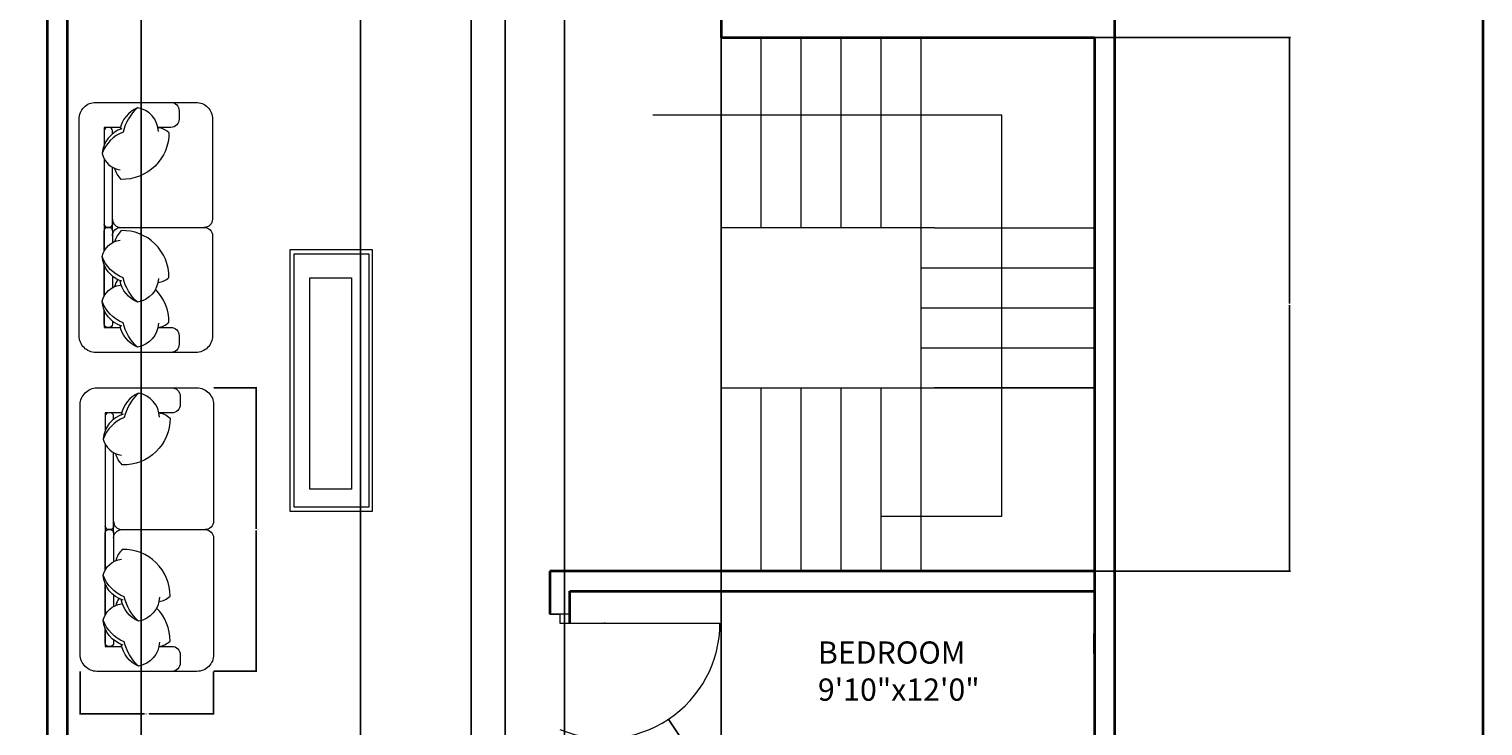
# Model space of a CAD drawing. Units: inches. Extents: x 1734 to 2405, y 1500 to 2491.
# Tile 10 of 14: x 2078 to 2405, y 1922 to 2078. Entities that reach past the tile are written whole.
import ezdxf

# ---------------------------------------------------------------- set-up
doc = ezdxf.new("R2010")
doc.units = ezdxf.units.IN
for name, color, linetype, lineweight in [('A-ANNO-DIMS', 2, 'Continuous', 18), ('A-ANNO-TTLB', 7, 'Continuous', 35), ('A-AREA-IDEN', 7, 'Continuous', 18), ('A-DOOR', 3, 'Continuous', 18), ('A-FLOR-STRS', 7, 'Continuous', 18), ('A-FURN', 8, 'Continuous', 13), ('A-WALL', 7, 'Continuous', 35)]:
    doc.layers.add(name, color=color, linetype=linetype, lineweight=lineweight)
doc.styles.get("Standard").update_dxf_attribs({"font": 'arial.ttf'})
doc.dimstyles.get("Standard").update_dxf_attribs({"dimtxt": 0.18, "dimasz": 0.18, "dimexe": 0.18, "dimexo": 0.0625, "dimgap": 0.09, "dimtad": 0, "dimtih": 1, "dimtoh": 1, "dimdec": 4, "dimzin": 0, "dimdsep": 46, "dimtxsty": 'Standard', "dimcen": 0.09, "dimadec": 0, "dimazin": 0, "dimtfac": 1, "dimtdec": 4, "dimtofl": 0, "dimtmove": 0, "dimatfit": 3, "dimfxl": 1, "dimtolj": 1, "dimtzin": 0, "dimarcsym": 0})

# ---------------------------------------------------------------- blocks, each defined once
blk = doc.blocks.new('SOFA-COMPACT')
at = {"ltscale": 0.03}
blk.add_lwpolyline([(29.99, 29.99, -0.414214), (28.12, 28.12, -0.414214), (29.99, 26.24), (29.99, 3.75, -0.414214), (26.24, 0), (3.75, 0, -0.414214), (0, 3.75), (0, 52.49, -0.414214), (3.75, 56.24), (26.24, 56.24, -0.414214), (29.99, 52.49), (29.99, 29.99, -0.414214), (28.12, 28.12, -0.414214), (29.99, 26.24)], format="xyb", dxfattribs=at)
for points in [[(20.62, 56.24, -0.414214), (22.49, 54.36), (22.49, 52.49, -0.414214), (20.62, 50.61), (17.72, 50.61)], [(13.1, 55.04, 0.14773), (9.88, 49.56, 0.213343), (5.16, 44.73, 0.178662)], [(17.83, 49.67, 0.356772), (13.1, 55.04, 0.249542), (9.21, 50.18, -9.61688)], [(9.63, 50.32, 0.306663), (5.16, 44.73, 0.30633), (9.24, 41.08, -0.872847)], [(7.5, 49.18), (7.5, 49.86, 0.414214), (6.75, 50.61), (6.37, 50.61, 0.414214), (5.62, 49.86)], [(5.62, 49.86), (5.62, 46.67, 0.414214)], [(17.71, 50.62, -0.165541), (20.19, 49.46, -0.425989), (9.45, 38.93, -0.121523), (7.97, 41.43, 7.115464)], [(5.62, 43.55), (5.62, 28.87, 0.414214), (6.37, 28.12), (6.75, 28.12, 0.414214), (7.5, 28.87), (7.5, 41.66, 0.414214)], [(7.5, 29.99, 0.414214), (9.37, 28.12)], [(7.5, 29.99, 0.414214), (9.37, 28.12), (28.12, 28.12, 0.414214)], [(5.62, 22.78), (5.62, 27.37, -0.414214), (6.37, 28.12), (6.75, 28.12, -0.414214), (7.5, 27.37), (7.5, 24.67, -0.414214)], [(7.5, 26.24, -0.414214), (9.37, 28.12)], [(7.5, 26.24, -0.414214), (9.37, 28.12), (28.12, 28.12, -0.414214)], [(17.71, 15.72, 0.165541), (20.19, 16.88, 0.425989), (9.45, 27.4, 0.121523), (7.97, 24.91, -7.115464)], [(9.63, 16.01, -0.306663), (5.16, 21.6, -0.30633), (9.24, 25.26, 0.872847)], [(13.1, 11.29, -0.14773), (9.88, 16.77, -0.213343), (5.16, 21.6, -0.178662)], [(5.62, 12.69), (5.62, 19.67, -0.414214)], [(7.5, 17.15), (7.5, 14.57, -0.414214)], [(8.71, 16.38, 0.071865), (7.97, 14.81, -7.115464)], [(17.83, 16.66, -0.356772), (13.1, 11.29, -0.249542), (9.21, 16.16, 9.61688)], [(9.63, 5.91, -0.306663), (5.16, 11.51, -0.30633), (9.24, 15.16, 0.872847)], [(17.71, 5.62, 0.165541), (20.19, 6.78, 0.200231), (17.17, 14.22, 0.121523)], [(13.1, 1.19, -0.14773), (9.88, 6.67, -0.213343), (5.16, 11.51, -0.178662)], [(5.62, 6.37), (5.62, 9.57, -0.414214)], [(5.62, 9.57), (5.62, 5.62), (9.31, 5.62, -0.414214)], [(7.5, 7.05), (7.5, 6.37, -0.414214), (6.75, 5.62), (6.37, 5.62, -0.414214), (5.62, 6.37)], [(17.83, 6.56, -0.356772), (13.1, 1.19, -0.249542), (9.21, 6.06, 9.61688)], [(17.72, 5.62), (20.62, 5.62, -0.414214), (22.49, 3.75), (22.49, 1.87, -0.414214), (20.62, 0)]]:
    blk.add_lwpolyline(points, format="xyb")
for points in [[(9.31, 50.61), (5.62, 50.61), (5.62, 46.67)], [(5.62, 43.55), (5.62, 22.78)], [(5.62, 19.67), (5.62, 12.69)]]:
    blk.add_lwpolyline(points)
blk.add_lwpolyline([(5.62, 28.87), (5.62, 27.37, -0.414214), (6.37, 28.12), (6.75, 28.12, -0.414214), (7.5, 27.37), (7.5, 28.87, -0.414214), (6.75, 28.12), (6.37, 28.12, -0.414214)], format="xyb", close=True)
blk = doc.blocks.new('SOFA-LONG')
at = {"ltscale": 0.03}
blk.add_lwpolyline([(29.99, 33.74, -0.414214), (28.12, 31.87, -0.414214), (29.99, 29.99), (29.99, 3.75, -0.414214), (26.24, 0), (3.75, 0, -0.414214), (0, 3.75), (0, 59.98, -0.414214), (3.75, 63.73), (26.24, 63.73, -0.414214), (29.99, 59.98), (29.99, 33.74, -0.414214), (28.12, 31.87, -0.414214), (29.99, 29.99)], format="xyb", dxfattribs=at)
for points in [[(13.1, 62.54, 0.14773), (9.88, 57.06, 0.213343), (5.16, 52.23, 0.178662)], [(17.83, 57.17, 0.356772), (13.1, 62.54, 0.249542), (9.21, 57.67, -9.61688)], [(20.62, 63.73, -0.414214), (22.49, 61.86), (22.49, 59.98, -0.414214), (20.62, 58.11), (17.71, 58.11)], [(9.63, 57.82, 0.306663), (5.16, 52.23, 0.30633), (9.24, 48.58, -0.872847)], [(7.5, 56.68), (7.5, 57.36, 0.414214), (6.75, 58.11), (6.37, 58.11, 0.414214), (5.62, 57.36)], [(5.62, 57.36), (5.62, 54.17, 0.414214)], [(17.71, 58.11, -0.165541), (20.19, 56.95, -0.425989), (9.45, 46.43, -0.121523), (7.97, 48.93, 7.115464)], [(5.62, 51.05), (5.62, 32.62, 0.414214), (6.37, 31.87), (6.75, 31.87, 0.414214), (7.5, 32.62), (7.5, 49.16, 0.414214)], [(7.5, 33.74, 0.414214), (9.37, 31.87)], [(7.5, 33.74, 0.414214), (9.37, 31.87), (28.12, 31.87, 0.414214)], [(5.62, 22.78), (5.62, 31.12, -0.414214), (6.37, 31.87), (6.75, 31.87, -0.414214), (7.5, 31.12), (7.5, 24.67, -0.414214)], [(7.5, 29.99, -0.414214), (9.37, 31.87)], [(7.5, 29.99, -0.414214), (9.37, 31.87), (28.12, 31.87, -0.414214)], [(17.71, 15.72, 0.165541), (20.19, 16.88, 0.425989), (9.45, 27.4, 0.121523), (7.97, 24.91, -7.115464)], [(9.63, 16.01, -0.306663), (5.16, 21.6, -0.30633), (9.24, 25.26, 0.872847)], [(13.1, 11.29, -0.14773), (9.88, 16.77, -0.213343), (5.16, 21.6, -0.178662)], [(5.62, 12.69), (5.62, 19.67, -0.414214)], [(7.5, 17.15), (7.5, 14.57, -0.414214)], [(8.71, 16.38, 0.071865), (7.97, 14.81, -7.115464)], [(17.83, 16.66, -0.356772), (13.1, 11.29, -0.249542), (9.21, 16.16, 9.61688)], [(9.63, 5.92, -0.306663), (5.16, 11.51, -0.30633), (9.24, 15.16, 0.872847)], [(17.71, 5.62, 0.165541), (20.19, 6.78, 0.200231), (17.17, 14.22, 0.121523)], [(13.1, 1.19, -0.14773), (9.88, 6.67, -0.213343), (5.16, 11.51, -0.178662)], [(5.62, 9.57), (5.62, 5.62), (9.31, 5.62, -0.414214)], [(5.62, 6.37), (5.62, 9.57, -0.414214)], [(7.5, 7.05), (7.5, 6.37, -0.414214), (6.75, 5.62), (6.37, 5.62, -0.414214), (5.62, 6.37)], [(17.83, 6.56, -0.356772), (13.1, 1.19, -0.249542), (9.21, 6.06, 9.61688)], [(17.71, 5.62), (20.62, 5.62, -0.414214), (22.49, 3.75), (22.49, 1.87, -0.414214), (20.62, 0)]]:
    blk.add_lwpolyline(points, format="xyb")
for points in [[(9.31, 58.11), (5.62, 58.11), (5.62, 54.17)], [(5.62, 51.05), (5.62, 22.78)], [(5.62, 19.67), (5.62, 12.69)]]:
    blk.add_lwpolyline(points)
blk.add_lwpolyline([(5.62, 32.62), (5.62, 31.12, -0.414214), (6.37, 31.87), (6.75, 31.87, -0.414214), (7.5, 31.12), (7.5, 32.62, -0.414214), (6.75, 31.87), (6.37, 31.87, -0.414214)], format="xyb", close=True)
blk = doc.blocks.new('TABLE-COFFEE')
for points in [[(0, 58.87), (18.49, 58.87), (18.49, 0), (0, 0)], [(0.91, 57.96), (17.71, 57.96), (17.71, 0.97), (0.91, 0.97)], [(4.43, 52.52), (13.86, 52.52), (13.86, 5), (4.43, 5)]]:
    blk.add_lwpolyline(points, close=True)
blk = doc.blocks.new('*D14')
at = {"layer": 'A-ANNO-DIMS', "color": 0, "lineweight": -2, "transparency": 16777216}
for p, q in [((2119.21, 1997.52), (2128.88, 1997.52)), ((2128.7, 1997.34), (2128.7, 1965.84)), ((2128.7, 1933.97), (2128.7, 1965.47)), ((2119.21, 1933.79), (2128.88, 1933.79))]:
    blk.add_line(p, q, dxfattribs=at)
at = {"layer": 'A-ANNO-DIMS', "color": 0, "transparency": 16777216}
for points in [[(2128.67, 1997.34), (2128.73, 1997.34), (2128.7, 1997.52)], [(2128.67, 1933.97), (2128.73, 1933.97), (2128.7, 1933.79)]]:
    blk.add_solid(points, dxfattribs=at)
at = {"layer": 'Defpoints', "color": 0, "transparency": 16777216}
for p in [(2119.14, 1997.52), (2128.7, 1997.52), (2119.14, 1933.79)]:
    blk.add_point(p, dxfattribs=at)
at = {"layer": 'A-ANNO-DIMS', "color": 0, "transparency": 16777216, "insert": (2128.7, 1965.65), "char_height": 0.18, "attachment_point": 5}
blk.add_mtext('\\A1;SOFA 64 TYP.', dxfattribs=at)
blk = doc.blocks.new('*D15')
at = {"layer": 'A-ANNO-DIMS', "color": 0, "lineweight": -2, "transparency": 16777216}
for p, q in [((2089.15, 1933.73), (2089.15, 1924.05)), ((2119.14, 1933.73), (2119.14, 1924.05)), ((2089.33, 1924.23), (2103.62, 1924.23)), ((2118.96, 1924.23), (2104.68, 1924.23))]:
    blk.add_line(p, q, dxfattribs=at)
at = {"layer": 'A-ANNO-DIMS', "color": 0, "transparency": 16777216}
for points in [[(2089.33, 1924.26), (2089.33, 1924.2), (2089.15, 1924.23)], [(2118.96, 1924.26), (2118.96, 1924.2), (2119.14, 1924.23)]]:
    blk.add_solid(points, dxfattribs=at)
at = {"layer": 'Defpoints', "color": 0, "transparency": 16777216}
for p in [(2089.15, 1933.79), (2119.14, 1933.79), (2119.14, 1924.23)]:
    blk.add_point(p, dxfattribs=at)
at = {"layer": 'A-ANNO-DIMS', "color": 0, "transparency": 16777216, "insert": (2104.15, 1924.23), "char_height": 0.18, "attachment_point": 5}
blk.add_mtext('\\A1;30 TYP.', dxfattribs=at)
blk = doc.blocks.new('*D36')
at = {"layer": 'A-ANNO-DIMS', "color": 0, "lineweight": -2, "transparency": 16777216}
for p, q in [((2081.68, 2425.82), (2042.21, 2425.82)), ((2042.39, 2425.64), (2042.39, 2065.96)), ((2042.39, 1705.92), (2042.39, 2065.6)), ((2081.68, 1705.74), (2042.21, 1705.74))]:
    blk.add_line(p, q, dxfattribs=at)
at = {"layer": 'A-ANNO-DIMS', "color": 0, "transparency": 16777216}
for points in [[(2042.36, 2425.64), (2042.42, 2425.64), (2042.39, 2425.82)], [(2042.36, 1705.92), (2042.42, 1705.92), (2042.39, 1705.74)]]:
    blk.add_solid(points, dxfattribs=at)
at = {"layer": 'Defpoints', "color": 0, "transparency": 16777216}
for p in [(2042.39, 2425.82), (2081.74, 2425.82), (2081.74, 1705.74)]:
    blk.add_point(p, dxfattribs=at)
at = {"layer": 'A-ANNO-DIMS', "color": 0, "transparency": 16777216, "insert": (2042.39, 2065.78), "char_height": 0.18, "attachment_point": 5}
blk.add_mtext('\\A1;720.1', dxfattribs=at)
blk = doc.blocks.new('*D39')
at = {"layer": 'A-ANNO-DIMS', "color": 0, "lineweight": -2, "transparency": 16777216}
for p, q in [((2317.31, 2076.32), (2361.27, 2076.32)), ((2361.09, 2076.14), (2361.09, 2016.51)), ((2361.09, 1956.5), (2361.09, 2016.14)), ((2317.31, 1956.32), (2361.27, 1956.32))]:
    blk.add_line(p, q, dxfattribs=at)
at = {"layer": 'A-ANNO-DIMS', "color": 0, "transparency": 16777216}
for points in [[(2361.06, 2076.14), (2361.12, 2076.14), (2361.09, 2076.32)], [(2361.06, 1956.5), (2361.12, 1956.5), (2361.09, 1956.32)]]:
    blk.add_solid(points, dxfattribs=at)
at = {"layer": 'Defpoints', "color": 0, "transparency": 16777216}
for p in [(2317.24, 2076.32), (2361.09, 2076.32), (2317.24, 1956.32)]:
    blk.add_point(p, dxfattribs=at)
at = {"layer": 'A-ANNO-DIMS', "color": 0, "transparency": 16777216, "insert": (2361.09, 2016.32), "char_height": 0.18, "attachment_point": 5}
blk.add_mtext('\\A1;120', dxfattribs=at)
blk = doc.blocks.new('*D41')
at = {"layer": 'A-ANNO-DIMS', "color": 0, "lineweight": -2, "transparency": 16777216}
for p, q in [((2233.24, 1956.26), (2233.24, 1611.24)), ((2317.24, 1956.26), (2317.24, 1611.24)), ((2233.42, 1611.42), (2275.03, 1611.42)), ((2317.06, 1611.42), (2275.46, 1611.42))]:
    blk.add_line(p, q, dxfattribs=at)
at = {"layer": 'A-ANNO-DIMS', "color": 0, "transparency": 16777216}
for points in [[(2233.42, 1611.45), (2233.42, 1611.39), (2233.24, 1611.42)], [(2317.06, 1611.45), (2317.06, 1611.39), (2317.24, 1611.42)]]:
    blk.add_solid(points, dxfattribs=at)
at = {"layer": 'Defpoints', "color": 0, "transparency": 16777216}
for p in [(2233.24, 1956.32), (2317.24, 1956.32), (2317.24, 1611.42)]:
    blk.add_point(p, dxfattribs=at)
at = {"layer": 'A-ANNO-DIMS', "color": 0, "transparency": 16777216, "insert": (2275.24, 1611.42), "char_height": 0.18, "attachment_point": 5}
blk.add_mtext('\\A1;84', dxfattribs=at)
blk = doc.blocks.new('*D42')
at = {"layer": 'A-ANNO-DIMS', "color": 0, "lineweight": -2, "transparency": 16777216}
for p, q in [((2152.2, 2198.26), (2152.2, 1611.24)), ((2184.72, 2198.26), (2184.72, 1611.24)), ((2152.38, 1611.42), (2168, 1611.42)), ((2184.54, 1611.42), (2168.92, 1611.42))]:
    blk.add_line(p, q, dxfattribs=at)
at = {"layer": 'A-ANNO-DIMS', "color": 0, "transparency": 16777216}
for points in [[(2152.38, 1611.45), (2152.38, 1611.39), (2152.2, 1611.42)], [(2184.54, 1611.45), (2184.54, 1611.39), (2184.72, 1611.42)]]:
    blk.add_solid(points, dxfattribs=at)
at = {"layer": 'Defpoints', "color": 0, "transparency": 16777216}
for p in [(2152.2, 2198.32), (2184.72, 2198.32), (2184.72, 1611.42)]:
    blk.add_point(p, dxfattribs=at)
at = {"layer": 'A-ANNO-DIMS', "color": 0, "transparency": 16777216, "insert": (2168.46, 1611.42), "char_height": 0.18, "attachment_point": 5}
blk.add_mtext('\\A1;32.526', dxfattribs=at)
blk = doc.blocks.new('*D43')
at = {"layer": 'A-ANNO-DIMS', "color": 0, "lineweight": -2, "transparency": 16777216}
for p, q in [((2233.24, 2200.45), (2233.24, 1611.24)), ((2198.08, 2198.26), (2198.08, 1611.24)), ((2198.26, 1611.42), (2215.27, 1611.42)), ((2233.06, 1611.42), (2216.05, 1611.42))]:
    blk.add_line(p, q, dxfattribs=at)
at = {"layer": 'A-ANNO-DIMS', "color": 0, "transparency": 16777216}
for points in [[(2198.26, 1611.45), (2198.26, 1611.39), (2198.08, 1611.42)], [(2233.06, 1611.45), (2233.06, 1611.39), (2233.24, 1611.42)]]:
    blk.add_solid(points, dxfattribs=at)
at = {"layer": 'Defpoints', "color": 0, "transparency": 16777216}
for p in [(2233.24, 2200.51), (2198.08, 2198.32), (2233.24, 1611.42)]:
    blk.add_point(p, dxfattribs=at)
at = {"layer": 'A-ANNO-DIMS', "color": 0, "transparency": 16777216, "insert": (2215.66, 1611.42), "char_height": 0.18, "attachment_point": 5}
blk.add_mtext('\\A1;35.17', dxfattribs=at)
blk = doc.blocks.new('*D44')
at = {"layer": 'A-ANNO-DIMS', "color": 0, "lineweight": -2, "transparency": 16777216}
for p, q in [((2102.87, 2356.76), (2102.87, 1611.24)), ((2177.04, 2356.76), (2177.04, 1611.24)), ((2103.05, 1611.42), (2139.56, 1611.42)), ((2176.86, 1611.42), (2140.35, 1611.42))]:
    blk.add_line(p, q, dxfattribs=at)
at = {"layer": 'A-ANNO-DIMS', "color": 0, "transparency": 16777216}
for points in [[(2103.05, 1611.45), (2103.05, 1611.39), (2102.87, 1611.42)], [(2176.86, 1611.45), (2176.86, 1611.39), (2177.04, 1611.42)]]:
    blk.add_solid(points, dxfattribs=at)
at = {"layer": 'Defpoints', "color": 0, "transparency": 16777216}
for p in [(2102.87, 2356.82), (2177.04, 2356.82), (2177.04, 1611.42)]:
    blk.add_point(p, dxfattribs=at)
at = {"layer": 'A-ANNO-DIMS', "color": 0, "transparency": 16777216, "insert": (2139.96, 1611.42), "char_height": 0.18, "attachment_point": 5}
blk.add_mtext('\\A1;74.17', dxfattribs=at)
blk = doc.blocks.new('*D50')
at = {"layer": 'A-ANNO-DIMS', "color": 0, "lineweight": -2, "transparency": 16777216}
for p, q in [((2206.97, 1944.63), (2207.15, 1944.63)), ((2207.06, 1944.54), (2207.06, 1944.72)), ((2230.01, 1910.06), (2221.5, 1922.88)), ((2230.19, 1910.06), (2230.01, 1910.06))]:
    blk.add_line(p, q, dxfattribs=at)
at = {"layer": 'A-ANNO-DIMS', "color": 0, "transparency": 16777216}
blk.add_solid([(2221.53, 1922.89), (2221.48, 1922.86), (2221.4, 1923.03)], dxfattribs=at)
at = {"layer": 'Defpoints', "color": 0, "transparency": 16777216}
for p in [(2207.06, 1944.63), (2221.4, 1923.03)]:
    blk.add_point(p, dxfattribs=at)
at = {"layer": 'A-ANNO-DIMS', "color": 0, "transparency": 16777216, "insert": (2230.67, 1910.06), "char_height": 0.18, "attachment_point": 5}
blk.add_mtext('\\A1;R25.93', dxfattribs=at)

msp = doc.modelspace()

# ---------------------------------------------------------------- linework, layer by layer
at = {"layer": 'A-ANNO-TTLB'}
msp.add_lwpolyline([(1734.1307, 2491.1293), (2404.5589, 2491.1293), (2404.5589, 1500.293), (1734.1307, 1500.293)], close=True, dxfattribs=at)
at = {"layer": 'A-DOOR'}
for p, q in [((2199.2445, 1946.6313), (2194.7445, 1946.6313)), ((2194.7445, 1946.6313), (2196.9945, 1946.6313)), ((2196.9945, 1946.6313), (2196.9945, 1944.6313)), ((2196.9945, 1944.6313), (2232.9945, 1944.6313))]:
    msp.add_line(p, q, dxfattribs=at)
msp.add_arc((2207.0621, 1944.6313), 25.9324, 247.155856, 0, dxfattribs=at)
at = {"layer": 'A-FLOR-STRS'}
for p, q in [((2233.2445, 2033.5364), (2233.2445, 2076.3246)), ((2242.2445, 2033.5364), (2242.2445, 2076.3246)), ((2251.2445, 2033.5364), (2251.2445, 2076.3246)), ((2260.2445, 2033.5364), (2260.2445, 2076.3246)), ((2269.2445, 2033.5364), (2269.2445, 2076.3246)), ((2278.2445, 2033.5364), (2278.2445, 2076.3246)), ((2217.8883, 2058.9549), (2296.2999, 2058.9549)), ((2296.2999, 2058.9549), (2296.2999, 1968.6387)), ((2281.2445, 2033.5364), (2233.2445, 2033.5364)), ((2278.2445, 1956.3246), (2278.2445, 2033.5364)), ((2281.2445, 2033.5364), (2317.2445, 2033.5364)), ((2278.2445, 2024.5364), (2317.2445, 2024.5364)), ((2278.2445, 2015.5364), (2317.2445, 2015.5364)), ((2278.2445, 2006.5364), (2317.2445, 2006.5364)), ((2233.2445, 1997.5364), (2233.2445, 1956.3246)), ((2233.2445, 1961.5364), (2233.2445, 1997.5364)), ((2233.2445, 1997.5364), (2317.2445, 1997.5364)), ((2242.2445, 1956.3246), (2242.2445, 1997.5364)), ((2251.2445, 1956.3246), (2251.2445, 1997.5364)), ((2260.2445, 1956.3246), (2260.2445, 1997.5364)), ((2269.2445, 1956.3246), (2269.2445, 1997.5364)), ((2317.2445, 1997.5364), (2281.2445, 1997.5364)), ((2296.2999, 1968.6387), (2269.2445, 1968.6387))]:
    msp.add_line(p, q, dxfattribs=at)
at = {"layer": 'A-WALL'}
for p, q in [((2081.7445, 2425.8246), (2081.7445, 1705.7415)), ((2321.7445, 2425.8246), (2321.7445, 1922.2954)), ((2086.2445, 2198.3246), (2086.2445, 1900.8246)), ((2233.2445, 2080.8246), (2233.2445, 2076.3246)), ((2233.2445, 2076.3246), (2237.7445, 2076.3246)), ((2237.7445, 2076.3246), (2317.2445, 2076.3246)), ((2317.2445, 2076.3246), (2317.2445, 1807.8246)), ((2317.2445, 2076.3246), (2317.2445, 2067.8246)), ((2317.2445, 2076.3246), (2317.2445, 2067.8246)), ((2199.2445, 1956.3246), (2194.7445, 1956.3246)), ((2194.7445, 1956.3246), (2194.7445, 1946.6313)), ((2317.2445, 1956.3246), (2199.2445, 1956.3246)), ((2199.2445, 1951.8246), (2317.2445, 1951.8246)), ((2199.2445, 1944.6313), (2199.2445, 1951.8246)), ((2317.2445, 1937.8246), (2317.2445, 1942.3246)), ((2321.7445, 1922.2954), (2321.7445, 1798.8246))]:
    msp.add_line(p, q, dxfattribs=at)

# ---------------------------------------------------------------- block references
at = {"layer": 'A-FURN'}
for name, p in [('SOFA-COMPACT', (2088.9007, 2005.4886)), ('TABLE-COFFEE', (2136.3236, 1969.7433)), ('SOFA-LONG', (2089.1527, 1933.7876))]:
    msp.add_blockref(name, p, dxfattribs=at)

# ---------------------------------------------------------------- texts
at = {"layer": 'A-AREA-IDEN', "insert": (2255.0202, 1940.5132), "char_height": 5, "attachment_point": 1}
msp.add_mtext_dynamic_manual_height_columns('BEDROOM\\P9\'10"x12\'0"', width=100.655825, gutter_width=12.5, heights=[0], dxfattribs=at)

# ---------------------------------------------------------------- dimensions: what is measured, and where the dimension line sits
at = {"layer": 'A-ANNO-DIMS'}
for base, p1, p2, override, picture, middle in [((2042.3945, 2425.8246), (2081.7445, 1705.7415), (2081.7445, 2425.8246), {"dimdec": 1, "dimlfac": 1, "dimrnd": 0, "dimzin": 0, "dimdsep": 46, "dimlunit": 2}, '*D36', (2042.3945, 2065.783)), ((2361.0945, 2076.3246), (2317.2445, 1956.3246), (2317.2445, 2076.3246), {"dimdec": 0, "dimlfac": 1, "dimrnd": 0, "dimzin": 0, "dimdsep": 46, "dimlunit": 2}, '*D39', (2361.0945, 2016.3246))]:
    dim = msp.add_linear_dim(base=base, p1=p1, p2=p2, angle=90, dimstyle='Standard', override=override, dxfattribs=at)
    dim.commit()
    dim.dimension.update_dxf_attribs({"geometry": picture, "text_midpoint": middle})
for base, p1, p2, override, picture, middle in [((2177.0411, 1611.4236), (2102.8692, 2356.8246), (2177.0411, 2356.8246), {"dimdec": 2, "dimlfac": 1, "dimrnd": 0, "dimzin": 0, "dimdsep": 46, "dimlunit": 2}, '*D44', (2139.9551, 1611.4236)), ((2233.2445, 1611.4236), (2198.0776, 2198.3246), (2233.2445, 2200.5102), {"dimdec": 2, "dimlfac": 1, "dimrnd": 0, "dimzin": 0, "dimdsep": 46, "dimlunit": 2}, '*D43', (2215.661, 1611.4236)), ((2184.7241, 1611.4236), (2152.1978, 2198.3246), (2184.7241, 2198.3246), {"dimdec": 3, "dimlfac": 1, "dimrnd": 0, "dimzin": 0, "dimdsep": 46, "dimlunit": 2}, '*D42', (2168.461, 1611.4236)), ((2317.2445, 1611.4236), (2233.2445, 1956.3246), (2317.2445, 1956.3246), {"dimdec": 0, "dimlfac": 1, "dimrnd": 0, "dimzin": 0, "dimdsep": 46, "dimlunit": 2}, '*D41', (2275.2445, 1611.4236))]:
    dim = msp.add_linear_dim(base=base, p1=p1, p2=p2, dimstyle='Standard', override=override, dxfattribs=at)
    dim.commit()
    dim.dimension.update_dxf_attribs({"geometry": picture, "text_midpoint": middle})
dim = msp.add_linear_dim(base=(2128.7043, 1997.5212), p1=(2119.1443, 1933.7881), p2=(2119.1443, 1997.5212), angle=90, text='SOFA <> TYP.', dimstyle='Standard', override={"dimdec": 0, "dimlfac": 1, "dimrnd": 0, "dimzin": 0, "dimdsep": 46, "dimlunit": 2}, dxfattribs=at)
dim.commit()
dim.dimension.update_dxf_attribs({"geometry": '*D14', "text_midpoint": (2128.7043, 1965.6547)})
dim = msp.add_radius_dim(center=(2207.0621, 1944.6313), mpoint=(2221.4048, 1923.0263), dimstyle='Standard', override={"dimdec": 2, "dimlfac": 1, "dimrnd": 0, "dimzin": 0, "dimdsep": 46, "dimlunit": 2}, dxfattribs=at)
dim.commit()
dim.dimension.update_dxf_attribs({"geometry": '*D50', "text_midpoint": (2230.6702, 1910.0633), "dimtype": 164})
dim = msp.add_linear_dim(base=(2119.1443, 1924.2281), p1=(2089.1522, 1933.7881), p2=(2119.1443, 1933.7881), text='<> TYP.', dimstyle='Standard', override={"dimdec": 0, "dimlfac": 1, "dimrnd": 0, "dimzin": 0, "dimdsep": 46, "dimlunit": 2}, dxfattribs=at)
dim.commit()
dim.dimension.update_dxf_attribs({"geometry": '*D15', "text_midpoint": (2104.1483, 1924.2281)})

doc.saveas('drawing.dxf')
